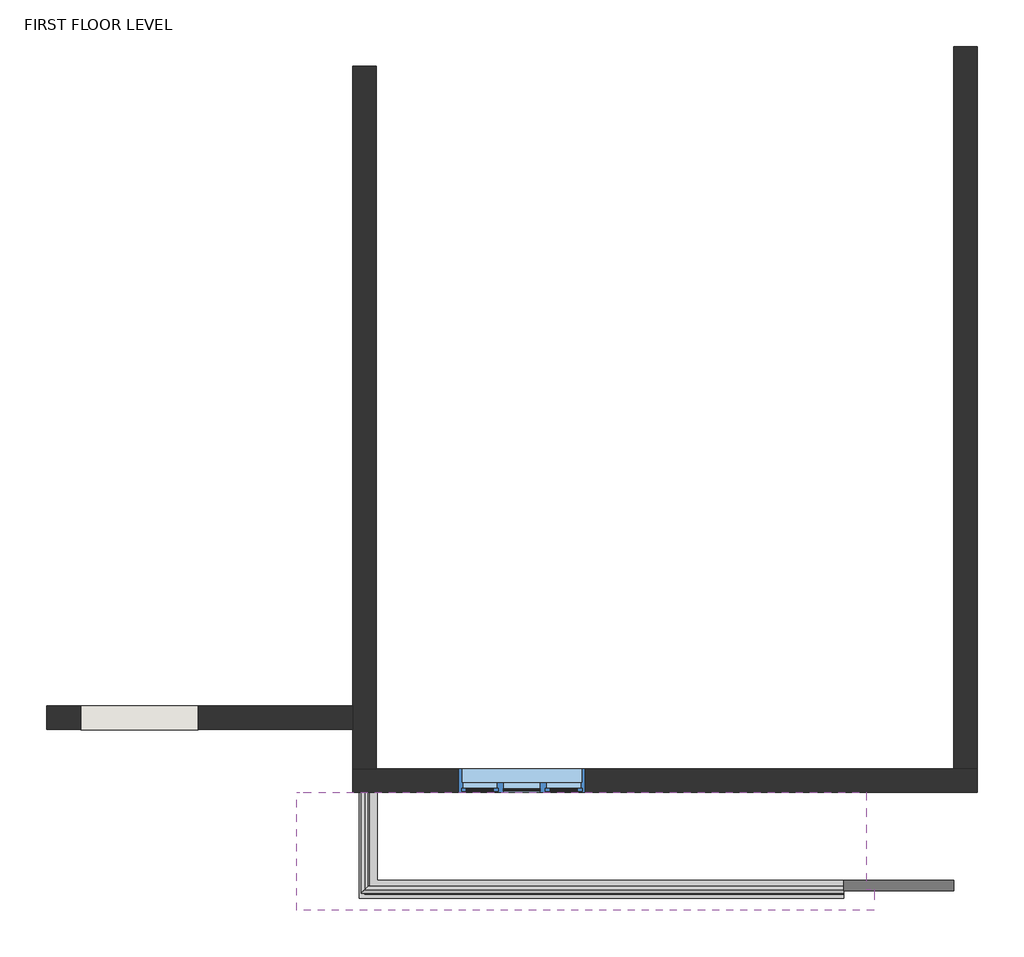
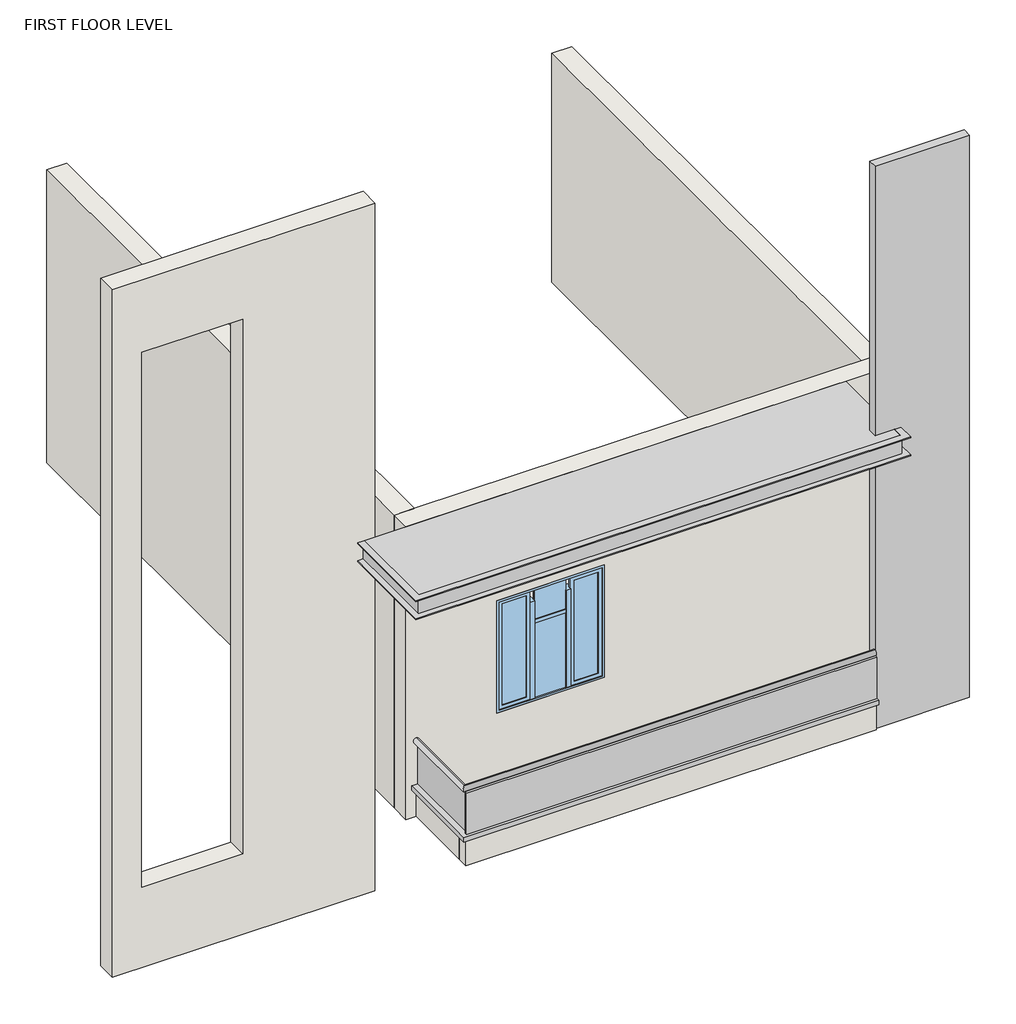
# One storey: 6 walls, 3 proxies, 2 members, 2 plates, 1 window.
"""IFC4 building model written with IfcOpenShell, lengths in millimetres."""

from ifc_helpers import new_model, si_unit, frame, origin, place, context, project, spatial, polyline, outline, extrude, faceted_brep, transform, mapped, element, save
from components import generic_models_4_generic_models_4_e8a7c7c6, generic_models_5_generic_models_5_f772a959, generic_models_6_generic_models_6_4d21afab, member_2ad469c0, member_72629bea, system_panel_glazed_e3058915, system_panel_glazed_6f34b03a, window_273a115f

model = new_model("IFC4")

# Units and contexts
model_context = context("Model", 3, world=origin())
ifc_project = project(units=[si_unit("LENGTHUNIT", "METRE", prefix="MILLI")], contexts=[model_context])

# Site, building, storey
site = spatial("IfcSite", under=ifc_project)
building = spatial("IfcBuilding", under=site)
storey = spatial("IfcBuildingStorey", under=building, Name="FIRST FLOOR LEVEL", Elevation=4419.6)

# Proxies
placement = place(None, origin())
generic_models_4_generic_models_4_shape = generic_models_4_generic_models_4_e8a7c7c6(model_context)
element("IfcBuildingElementProxy", 1, Name="Generic Models 4 : Generic Models 4", ObjectType="Generic Models 4 : Generic Models 4", at=placement, inside=storey, context=model_context, shape_type="MappedRepresentation", body=[
    mapped(generic_models_4_generic_models_4_shape, transform((0.0, 0.0, 0.0), x_axis=(1.0, 0.0, 0.0), y_axis=(0.0, 1.0, 0.0), z_axis=(0.0, 0.0, 1.0))),
])
generic_models_5_generic_models_5_shape = generic_models_5_generic_models_5_f772a959(model_context)
element("IfcBuildingElementProxy", 2, Name="Generic Models 5 : Generic Models 5", ObjectType="Generic Models 5 : Generic Models 5", at=placement, inside=storey, context=model_context, shape_type="MappedRepresentation", body=[
    mapped(generic_models_5_generic_models_5_shape, transform((0.0, 0.0, 0.0), x_axis=(1.0, 0.0, 0.0), y_axis=(0.0, 1.0, 0.0), z_axis=(0.0, 0.0, 1.0))),
])
generic_models_6_generic_models_6_shape = generic_models_6_generic_models_6_4d21afab(model_context)
element("IfcBuildingElementProxy", 3, Name="Generic Models 6 : Generic Models 6", ObjectType="Generic Models 6 : Generic Models 6", at=placement, inside=storey, context=model_context, shape_type="MappedRepresentation", body=[
    mapped(generic_models_6_generic_models_6_shape, transform((0.0, 0.0, 0.0), x_axis=(1.0, 0.0, 0.0), y_axis=(0.0, 1.0, 0.0), z_axis=(0.0, 0.0, 1.0))),
])

# Members
member_shape = member_2ad469c0(model_context)
element("IfcMember", 4, ObjectType="Circular Mullion : 2.5\" Circular", at=placement, inside=storey, context=model_context, shape_type="MappedRepresentation", body=[
    mapped(member_shape, transform((3233.2271331, -12920.3268494, 5359.4), x_axis=(0.0, 0.0, 1.0), y_axis=(0.0, 1.0, 0.0), z_axis=(-1.0, 0.0, 0.0))),
])
member_2_shape = member_72629bea(model_context)
element("IfcMember", 5, ObjectType="Circular Mullion : 2.5\" Circular", at=placement, inside=storey, context=model_context, shape_type="MappedRepresentation", body=[
    mapped(member_2_shape, transform((3233.2271331, -12920.3268494, 5359.4), x_axis=(0.0, 0.0, 1.0), y_axis=(-1.0, 0.0, 0.0), z_axis=(0.0, -1.0, 0.0))),
])

# Plates
system_panel_glazed_shape = system_panel_glazed_e3058915(model_context)
element("IfcPlate", 6, ObjectType="System Panel : Glazed", at=placement, inside=storey, context=model_context, shape_type="MappedRepresentation", body=[
    mapped(system_panel_glazed_shape, transform((3233.2271331, -12448.0455994, 4800.6), x_axis=(0.0, -1.0, 0.0), y_axis=(1.0, 0.0, 0.0), z_axis=(0.0, 0.0, 1.0))),
])
system_panel_glazed_2_shape = system_panel_glazed_6f34b03a(model_context)
element("IfcPlate", 7, ObjectType="System Panel : Glazed", at=placement, inside=storey, context=model_context, shape_type="MappedRepresentation", body=[
    mapped(system_panel_glazed_2_shape, transform((5557.3271331, -12920.3268494, 4800.6), x_axis=(-1.0, 0.0, 0.0), y_axis=(0.0, -1.0, 0.0), z_axis=(0.0, 0.0, 1.0))),
])

# Walls
element("IfcWall", 8, ObjectType="9\"", at=placement, inside=storey, context=model_context, shape_type="SweptSolid", body=[
    extrude(outline(polyline([(3200.4, 3118.9271331), (11430.0, 3118.9271331), (11430.0, 147.1271331), (3200.4, 147.1271331), (3200.4, 3118.9271331)]), holes=[polyline([(10566.4, 1620.3271331), (4165.6, 1620.3271331), (4165.6, 477.3271331), (10566.4, 477.3271331), (10566.4, 1620.3271331)])]), frame((0.0, -11366.1643494, 0.0), z_axis=(0.0, 1.0, 0.0), x_axis=(0.0, 0.0, 1.0)), (0.0, 0.0, 1.0), 228.6),
])
element("IfcWall", 9, ObjectType="9\"", at=placement, inside=storey, context=model_context, shape_type="Brep", body=[
    faceted_brep([(3118.9271331, -11975.7643494, 7924.8), (3118.9271331, -11975.7643494, 4419.6), (3233.2271331, -11975.7643494, 4419.6), (3357.0521331, -11975.7643494, 4419.6), (9176.8271331, -11975.7643494, 4419.6), (9176.8271331, -11975.7643494, 7924.8), (4147.6271331, -11975.7643494, 6680.2), (5366.8271331, -11975.7643494, 6680.2), (5366.8271331, -11975.7643494, 5334.0), (4147.6271331, -11975.7643494, 5334.0), (3118.9271331, -11747.1643494, 4419.6), (3118.9271331, -11747.1643494, 7924.8), (3347.5271331, -11747.1643494, 7924.8), (9176.8271331, -11747.1643494, 7924.8), (9176.8271331, -11747.1643494, 7162.8), (9176.8271331, -11747.1643494, 4419.6), (8948.2271331, -11747.1643494, 4419.6), (3347.5271331, -11747.1643494, 4419.6), (4147.6271331, -11747.1643494, 6680.2), (4147.6271331, -11747.1643494, 5334.0), (5366.8271331, -11747.1643494, 5334.0), (5366.8271331, -11747.1643494, 6680.2)], [[[0, 1, 2, 3, 4, 5], [6, 7, 8, 9]], [[10, 11, 12, 13, 14, 15, 16, 17], [18, 19, 20, 21]], [[4, 3, 2, 1, 10, 17, 16, 15]], [[0, 5, 13, 12, 11]], [[5, 4, 15, 14, 13]], [[19, 18, 6, 9]], [[20, 19, 9, 8]], [[21, 20, 8, 7]], [[18, 21, 7, 6]], [[0, 11, 10, 1]]]),
])
element("IfcWall", 10, ObjectType="9\"", at=placement, inside=storey, context=model_context, shape_type="SweptSolid", body=[
    extrude(outline(polyline([(3347.5271331, -4927.2643494), (3347.5271331, -11747.1643494), (3118.9271331, -11747.1643494), (3118.9271331, -4927.2643494), (3347.5271331, -4927.2643494)])), frame((0.0, 0.0, 4419.6), z_axis=(0.0, 0.0, 1.0), x_axis=(1.0, 0.0, 0.0)), (0.0, 0.0, 1.0), 3505.2),
])
element("IfcWall", 11, ObjectType="9\"", at=placement, inside=storey, context=model_context, shape_type="SweptSolid", body=[
    extrude(outline(polyline([(9176.8271331, -4736.7643494), (9176.8271331, -11747.1643494), (8948.2271331, -11747.1643494), (8948.2271331, -4736.7643494), (9176.8271331, -4736.7643494)])), frame((0.0, 0.0, 4419.6), z_axis=(0.0, 0.0, 1.0), x_axis=(1.0, 0.0, 0.0)), (0.0, 0.0, 1.0), 2743.2),
])
element("IfcWall", 12, ObjectType="Interior - 4 7/8\" Partition (1-hr)", at=placement, inside=storey, context=model_context, shape_type="Brep", body=[
    faceted_brep([(7881.4271331, -12826.6643494, 4419.6), (3357.0521331, -12826.6643494, 4419.6), (3233.2271331, -12826.6643494, 4419.6), (3233.2271331, -12826.6643494, 4749.8), (3357.0521331, -12826.6643494, 4749.8), (7881.4271331, -12826.6643494, 4749.8), (7881.4271331, -12950.4893494, 4419.6), (7881.4271331, -12950.4893494, 4749.8), (3233.2271331, -12950.4893494, 4749.8), (3233.2271331, -12950.4893494, 4419.6)], [[[0, 1, 2, 3, 4, 5]], [[6, 7, 8, 9]], [[2, 1, 0, 6, 9]], [[5, 4, 3, 8, 7]], [[0, 5, 7, 6]], [[3, 2, 9, 8]]]),
])
element("IfcWall", 13, ObjectType="Interior - 4 7/8\" Partition (1-hr)", at=placement, inside=storey, context=model_context, shape_type="SweptSolid", body=[
    extrude(outline(polyline([(3357.0521331, -11975.7643494), (3357.0521331, -12826.6643494), (3233.2271331, -12826.6643494), (3233.2271331, -11975.7643494), (3357.0521331, -11975.7643494)])), frame((0.0, 0.0, 4419.6), z_axis=(0.0, 0.0, 1.0), x_axis=(1.0, 0.0, 0.0)), (0.0, 0.0, 1.0), 330.2),
])

# Window
window_shape = window_273a115f(model_context)
element("IfcWindow", 14, ObjectType="Window-Casement-Triple-Middle-Transom : 48\" x 53\"", at=placement, inside=storey, context=model_context, shape_type="MappedRepresentation", body=[
    mapped(window_shape, transform((4757.2271331, -11861.4643494, 4419.6), x_axis=(-1.0, 0.0, 0.0), y_axis=(0.0, -1.0, 0.0), z_axis=(0.0, 0.0, 1.0))),
])

save(model, "model.ifc")

# Revit data of these elements
# Type "Circular Mullion : 2.5\" Circular"
#   built-in parameter 1007350 = 0.104167 (stored number, unit not read)
# Type "System Panel : Glazed"
#   Construction Type Id = "GSP4R"
#   Analytic Construction = "1/8 in Pilkington single glazing"
#   Visual Light Transmittance = 0.9
#   Solar Heat Gain Coefficient = 0.86
#   Heat Transfer Coefficient (U) = 1.18115 BTU/(h·ft²·°F)
#   Define Thermal Properties by = 1
# Type "9\""
#   Assembly Code = "B2010"
#   Layers, outside or top first: 0' - 9" no material (function 1)
# Type "Interior - 4 7/8\" Partition (1-hr)"
#   Assembly Code = "C1010145"
#   Layers, outside or top first: 0' - 0 5/8" "Gypsum Wall Board" (function 5); 0' - 3 5/8" "Metal Stud Layer" (function 1); 0' - 0 5/8" "Gypsum Wall Board" (function 5)
# Type "Window-Casement-Triple-Middle-Transom : 48\" x 53\""
#   Type Mark = "18"
#   Fire Rating = "0.5h"
#   Assembly Code = "B2020100"
#   Analytic Construction = "Double glazing - domestic"
#   Window Width = 1' - 4"
#   Window Inset [instance default] = 0' - 0 5/8"
#   Wall Thickness [instance default] = 0' - 6"
#   Visual Light Transmittance = 0.81
#   Transom Height Ratio = 0.3
#   Thermal Resistance (R) = 1.8146 (h·ft²·°F)/BTU
#   Solar Heat Gain Coefficient = 0.76
#   Rough Width = 4' - 0 1/2"
#   Rough Height = 4' - 5 1/2"
#   Heat Transfer Coefficient (U) = 0.5511 BTU/(h·ft²·°F)
#   Height = 4' - 5"
#   Transom Height = 1' - 3.9"
#   Frame Gap 3 [instance default] = 0' - 1 83/128"
#   Frame Gap 2 [instance default] = 0' - 0 5/8"
#   Frame Gap 1 = 0' - 1 51/128"
#   Default Sill Height = 3' - 0"
#   Width = 4' - 0"
#   Frame Material = Metal - Aluminum
#   Glass Panel Material = Glass
#   Wall Closure = (empty or 0)
# Element 1 (IfcBuildingElementProxy, "Generic Models 4 : Generic Models 4")
#   Phase Created = New Construction
# Element 2 (IfcBuildingElementProxy, "Generic Models 5 : Generic Models 5")
#   Phase Created = New Construction
# Element 3 (IfcBuildingElementProxy, "Generic Models 6 : Generic Models 6")
#   Phase Created = New Construction
# Elements 4, 5 (IfcMember, "Circular Mullion : 2.5\" Circular")
#   Phase Created = New Construction
#   Materials on its faces: "Aluminum"
# Elements 6, 7 (IfcPlate, "System Panel : Glazed")
#   Phase Created = New Construction
#   Materials on its faces: "Glass"
# Element 8 (IfcWall, "9\"")
#   built-in parameter 1001111 = -4' - 0"
#   Top Offset = 0' - 0"
#   Base Offset = -4' - 0"
#   wall height = 27' - 0"
#   Phase Created = New Construction
#   Base Constraint = FIRST FLOOR LEVEL
#   Top Constraint = ROOF LEVEL
#   Materials on its faces: "Default Wall"
# Element 9 (IfcWall, "9\"")
#   Top Offset = 0' - 0"
#   Base Offset = 0' - 0"
#   wall height = 11' - 6"
#   Phase Created = New Construction
#   Base Constraint = FIRST FLOOR LEVEL
#   Top Constraint = SECOND FLOOR LEVEL
#   Materials on its faces: "Default Wall"
# Element 10 (IfcWall, "9\"")
#   Top Offset = 0' - 0"
#   Base Offset = 0' - 0"
#   Unconnected Height = 11' - 6"
#   wall height = 11' - 6"
#   Phase Created = New Construction
#   Base Constraint = FIRST FLOOR LEVEL
#   Materials on its faces: "Default Wall"
# Element 11 (IfcWall, "9\"")
#   Top Offset = 0' - 0"
#   Base Offset = 0' - 0"
#   Unconnected Height = 9' - 0"
#   wall height = 9' - 0"
#   Phase Created = New Construction
#   Base Constraint = FIRST FLOOR LEVEL
#   Materials on its faces: "Default Wall"
# Element 12 (IfcWall, "Interior - 4 7/8\" Partition (1-hr)")
#   Top Offset = 0' - 0"
#   Base Offset = 0' - 0"
#   Unconnected Height = 1' - 1"
#   wall height = 1' - 1"
#   Phase Created = New Construction
#   Base Constraint = FIRST FLOOR LEVEL
#   Materials on its faces: "Gypsum Wall Board", "Default Wall"
# Element 13 (IfcWall, "Interior - 4 7/8\" Partition (1-hr)")
#   Top Offset = 0' - 0"
#   Base Offset = 0' - 0"
#   Unconnected Height = 1' - 1"
#   wall height = 1' - 1"
#   Phase Created = New Construction
#   Base Constraint = FIRST FLOOR LEVEL
#   Materials on its faces: "Default Wall", "Gypsum Wall Board"
# Element 14 (IfcWindow, "Window-Casement-Triple-Middle-Transom : 48\" x 53\"")
#   Mark = "4"
#   Window Inset = 0' - 0 5/8"
#   Frame Gap 3 = 0' - 1 83/128"
#   Frame Gap 2 = 0' - 0 5/8"
#   Phase Created = New Construction
#   Materials on its faces: "Metal - Aluminum", "Glass"
# Materials
#   "Gypsum Wall Board": class "Generic", colour RGB 228 228 228, transparency 0, Description = "Gypsum Wall Board", Cost = 0
#   "Metal Stud Layer": class "Metal", colour RGB 199 199 199, transparency 0, Description = "Light gauge steel framing, thermal air layer", Cost = 0
#   "Metal - Aluminum": class "Metal", colour RGB 247 247 247, transparency 0
#   "Glass": class "Glass", colour RGB 0 128 192, transparency 0.75, Description = "Soda Lime Glass", Cost = 0
#   "Aluminum": class "Metal", colour RGB 247 247 247, transparency 0, Description = "Aluminum 6061", Cost = 0
#   "Default Wall": colour RGB 128 128 128, transparency 0, Cost = 0
